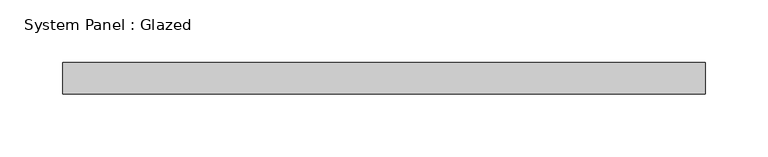
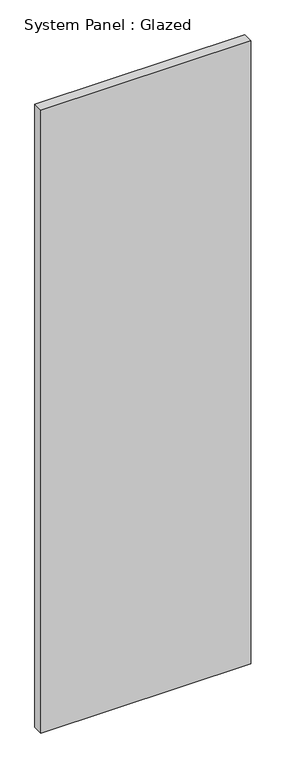
"""IFC4 building model written with IfcOpenShell, lengths in millimetres: plate geometry, System Panel : Glazed."""

from ifc_helpers import new_model, si_unit, origin, origin_with_axes, place, context, project, spatial, polyline, outline, extrude, source, transform, mapped, element, save


def system_panel_glazed_df895792(model_context):
    return source(origin(), model_context, "Body", "SweptSolid", [
        extrude(outline(polyline([(257.175, 19.05), (-257.175, 19.05), (-257.175, 44.45), (257.175, 44.45), (257.175, 19.05)])), origin_with_axes(), (0.0, 0.0, 1.0), 1614.7653418),
    ])


if __name__ == "__main__":
    model = new_model("IFC4")
    model_context = context("Model", 3, world=origin())
    ifc_project = project(units=[si_unit("LENGTHUNIT", "METRE", prefix="MILLI")], contexts=[model_context])
    site = spatial("IfcSite", under=ifc_project)
    building = spatial("IfcBuilding", under=site)
    placement = place(None, origin())
    system_panel_glazed_shape = system_panel_glazed_df895792(model_context)
    element("IfcPlate", 1, ObjectType="System Panel : Glazed", at=placement, inside=building, context=model_context, shape_type="MappedRepresentation", body=[
        mapped(system_panel_glazed_shape, transform((0.0, 0.0, 0.0), x_axis=(1.0, 0.0, 0.0), y_axis=(0.0, 1.0, 0.0), z_axis=(0.0, 0.0, 1.0))),
    ])
    save(model, "model.ifc")

# Revit data of these elements
# Type "System Panel : Glazed"
#   Construction Type Id = "GSP4R"
#   Analytic Construction = "1/8 in Pilkington single glazing"
#   Visual Light Transmittance = 0.9
#   Solar Heat Gain Coefficient = 0.86
#   Heat Transfer Coefficient (U) = 1.18115 BTU/(h·ft²·°F)
#   Define Thermal Properties by = 1
# Element 1 (IfcPlate, "System Panel : Glazed")
#   Materials on its faces: "Glass"
# Materials
#   "Glass": class "Glass", colour RGB 0 128 192, transparency 0.75, Description = "Soda Lime Glass", Cost = 0
